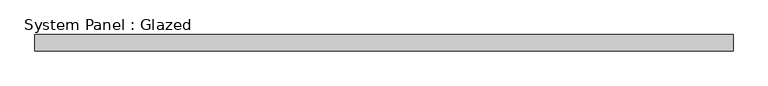
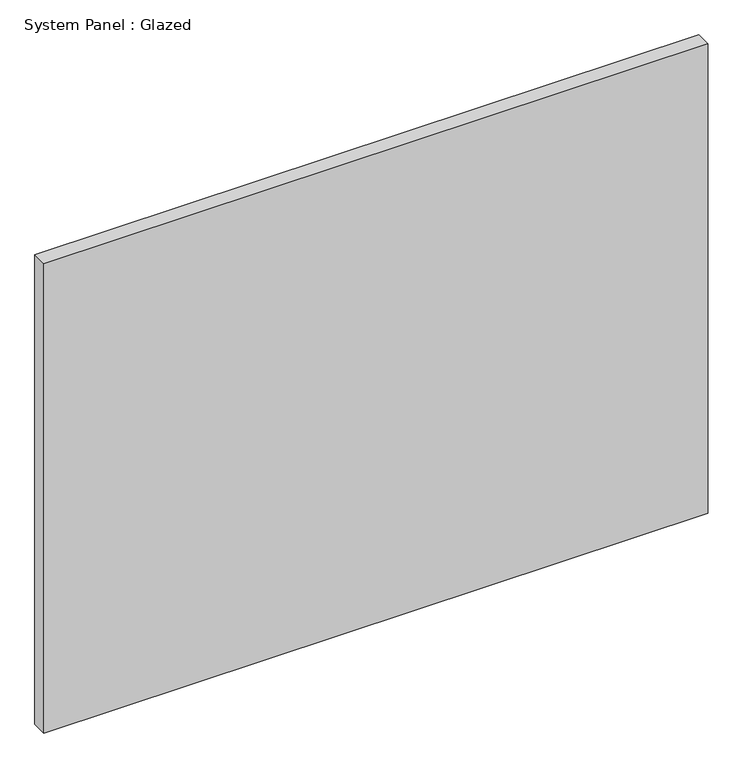
"""IFC4 building model written with IfcOpenShell, lengths in millimetres: plate geometry, System Panel : Glazed."""

from ifc_helpers import new_model, si_unit, origin, origin_with_axes, place, context, project, spatial, polyline, outline, extrude, source, transform, mapped, element, save


def system_panel_glazed_a48af828(model_context):
    return source(origin(), model_context, "Body", "SweptSolid", [
        extrude(outline(polyline([(549.2750001, 19.05), (-549.2750001, 19.05), (-549.2750001, 44.45), (549.2750001, 44.45), (549.2750001, 19.05)])), origin_with_axes(), (0.0, 0.0, 1.0), 820.4497825),
    ])


if __name__ == "__main__":
    model = new_model("IFC4")
    model_context = context("Model", 3, world=origin())
    ifc_project = project(units=[si_unit("LENGTHUNIT", "METRE", prefix="MILLI")], contexts=[model_context])
    site = spatial("IfcSite", under=ifc_project)
    building = spatial("IfcBuilding", under=site)
    placement = place(None, origin())
    system_panel_glazed_shape = system_panel_glazed_a48af828(model_context)
    element("IfcPlate", 1, ObjectType="System Panel : Glazed", at=placement, inside=building, context=model_context, shape_type="MappedRepresentation", body=[
        mapped(system_panel_glazed_shape, transform((0.0, 0.0, 0.0), x_axis=(1.0, 0.0, 0.0), y_axis=(0.0, 1.0, 0.0), z_axis=(0.0, 0.0, 1.0))),
    ])
    save(model, "model.ifc")

# Revit data of these elements
# Type "System Panel : Glazed"
#   Construction Type Id = "GSP4R"
#   Analytic Construction = "1/8 in Pilkington single glazing"
#   Visual Light Transmittance = 0.9
#   Solar Heat Gain Coefficient = 0.86
#   Heat Transfer Coefficient (U) = 1.18115 BTU/(h·ft²·°F)
#   Define Thermal Properties by = 1
# Element 1 (IfcPlate, "System Panel : Glazed")
#   Materials on its faces: "Glass"
# Materials
#   "Glass": class "Glass", colour RGB 0 128 192, transparency 0.75, Description = "Soda Lime Glass", Cost = 0
